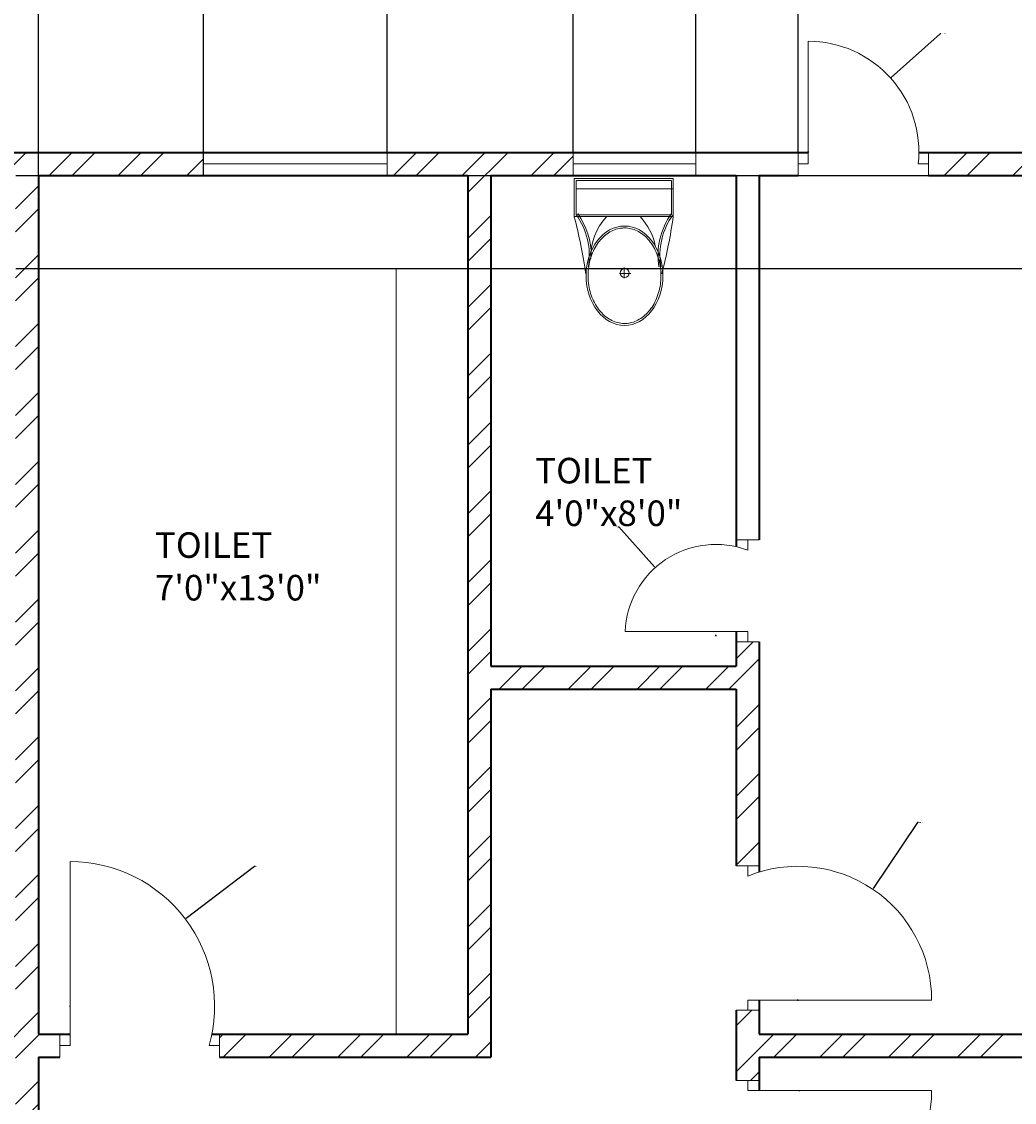
# Model space of a CAD drawing. Units: inches. Extents: x 392 to 1254, y 1207 to 2665.
# Tile 13 of 15: x 832 to 1026, y 2043 to 2255. Entities that reach past the tile are written whole.
import ezdxf

# ---------------------------------------------------------------- set-up
doc = ezdxf.new("R2010")
doc.units = ezdxf.units.IN
for name, color, linetype, lineweight in [('A-ANNO-DIMS', 2, 'Continuous', 18), ('A-AREA-IDEN', 7, 'Continuous', 18), ('A-DOOR', 3, 'Continuous', 18), ('A-FLOR-FIXT', 9, 'Continuous', 18), ('A-GLAZ', 4, 'Continuous', 18), ('A-WALL', 7, 'Continuous', 35), ('A-WALL-PATT', 252, 'Continuous', 13)]:
    doc.layers.add(name, color=color, linetype=linetype, lineweight=lineweight)
doc.styles.get("Standard").update_dxf_attribs({"font": 'arial.ttf'})
doc.dimstyles.get("Standard").update_dxf_attribs({"dimtxt": 0.18, "dimasz": 0.18, "dimexe": 0.18, "dimexo": 0.0625, "dimgap": 0.09, "dimtad": 0, "dimtih": 1, "dimtoh": 1, "dimdec": 4, "dimzin": 0, "dimdsep": 46, "dimtxsty": 'Standard', "dimcen": 0.09, "dimadec": 0, "dimazin": 0, "dimtfac": 1, "dimtdec": 4, "dimtofl": 0, "dimtmove": 0, "dimatfit": 3, "dimfxl": 1, "dimtolj": 1, "dimtzin": 0, "dimarcsym": 0})

# ---------------------------------------------------------------- blocks, each defined once
blk = doc.blocks.new('A$C31115884')
for p, q in [((257.5, 466.4), (257.5, 523.2)), ((283.1, 497.7), (223.4, 497.7)), ((0, 200), (0, 0)), ((520, 200), (0, 200)), ((10, 190), (10, 10)), ((510, 190), (10, 190)), ((510, 10), (510, 190)), ((520, 0), (520, 200)), ((510, 54.5), (0, 54.5)), ((10, 10), (510, 10)), ((0, 0), (520, 0))]:
    blk.add_line(p, q)
blk.add_circle((255.6, 496.4), 23.6)
for centre, radius, start, end in [((2777.7, -204.6), 2807, 165.4549, 171.7133), ((-294.5, 403.3), 364.7, 324.2091, 9.3499), ((-294.5, 403.3), 374.7, 324.2091, 9.3499), ((805.8, 403.3), 364.7, 170.6501, 215.7909), ((3237, 905), 2807, 188.2867, 194.5451), ((139.5, 406.2), 293.5, 315.8436, 2.6563), ((805.8, 403.3), 374.7, 179.2036, 215.7909), ((383.6, 406.2), 293.5, 190.2774, 224.1564)]:
    blk.add_arc(centre, radius, start, end)
blk.add_ellipse((256.2, 509.9), major_axis=(0, -260.7), ratio=0.772727)
blk.add_open_spline([(256.2, 259.2), (263.1, 259.2), (270, 259.7), (287.8, 262.3), (298.7, 265.1), (319.9, 273.1), (330.2, 278.4), (350.1, 291.1), (359.7, 298.7), (377.7, 315.9), (386.2, 325.5), (401.7, 346.6), (408.8, 358.1), (421.3, 382.5), (426.8, 395.5), (435.9, 422.4), (439.5, 436.4), (444.8, 465.1), (446.5, 479.7), (447.9, 509.2), (447.6, 524), (445, 553.3), (442.7, 567.8), (436.3, 596), (432.1, 609.7), (421.9, 636), (416, 648.6), (402.5, 672.1), (395, 683), (378.6, 703), (369.8, 712.1), (351.1, 728), (341.3, 734.8), (320.9, 746.2), (310.4, 750.7), (288.9, 757.3), (278, 759.4), (256, 761), (245, 760.6), (223.1, 757.2), (212.3, 754.3), (191.1, 746.1), (180.8, 740.7), (160.9, 727.8), (151.4, 720.1), (133.5, 702.7), (125.1, 693), (109.6, 671.7), (102.6, 660.2), (90.2, 635.7), (84.9, 622.7), (76, 595.6), (72.4, 581.6), (67.2, 552.9), (65.6, 538.2), (64.4, 508.8), (64.8, 494), (67.5, 464.7), (69.9, 450.2), (76.6, 422), (80.8, 408.3), (91.1, 382.2), (97.2, 369.7), (110.8, 346.3), (118.4, 335.4), (134.8, 315.6), (143.7, 306.7), (162.4, 290.9), (172.3, 284.2), (192.8, 273), (203.3, 268.6), (224.8, 262.2), (235.8, 260.2), (249.9, 259.3), (253, 259.2), (256.2, 259.2)], degree=3, knots=[0, 0, 0, 0, 0.110105, 0.110105, 0.285049, 0.285049, 0.459994, 0.459994, 0.634938, 0.634938, 0.809882, 0.809882, 0.984827, 0.984827, 1.159771, 1.159771, 1.334715, 1.334715, 1.50966, 1.50966, 1.684604, 1.684604, 1.859549, 1.859549, 2.034493, 2.034493, 2.209437, 2.209437, 2.384382, 2.384382, 2.559326, 2.559326, 2.73427, 2.73427, 2.909215, 2.909215, 3.084159, 3.084159, 3.259103, 3.259103, 3.434048, 3.434048, 3.608992, 3.608992, 3.783936, 3.783936, 3.958881, 3.958881, 4.133825, 4.133825, 4.30877, 4.30877, 4.483714, 4.483714, 4.658658, 4.658658, 4.833603, 4.833603, 5.008547, 5.008547, 5.183491, 5.183491, 5.358436, 5.358436, 5.53338, 5.53338, 5.708324, 5.708324, 5.883269, 5.883269, 6.058213, 6.058213, 6.233158, 6.233158, 6.283185, 6.283185, 6.283185, 6.283185])
blk = doc.blocks.new('WIN-24-A')
for p, q in [((0, 0), (0, 4.5)), ((0, 4.5), (0, 2.25)), ((24, 2.25), (24, 4.5)), ((24, 4.5), (24, 0)), ((0, 2.25), (24, 2.25))]:
    blk.add_line(p, q)
blk = doc.blocks.new('WIN-36')
for p, q in [((0, 0), (0, 4.5)), ((0, 4.5), (0, 2.25)), ((36, 2.25), (36, 4.5)), ((36, 4.5), (36, 0)), ((0, 2.25), (36, 2.25))]:
    blk.add_line(p, q)
blk = doc.blocks.new('*D47')
at = {"layer": 'A-ANNO-DIMS', "color": 0, "lineweight": -2, "transparency": 16777216}
for p, q in [((903.51, 2229.36), (903.51, 2297.33)), ((903.69, 2297.15), (921.29, 2297.15)), ((939.68, 2297.15), (922.08, 2297.15)), ((939.86, 2229.36), (939.86, 2297.33))]:
    blk.add_line(p, q, dxfattribs=at)
at = {"layer": 'A-ANNO-DIMS', "color": 0, "transparency": 16777216}
for points in [[(903.69, 2297.18), (903.69, 2297.12), (903.51, 2297.15)], [(939.68, 2297.18), (939.68, 2297.12), (939.86, 2297.15)]]:
    blk.add_solid(points, dxfattribs=at)
at = {"layer": 'Defpoints', "color": 0, "transparency": 16777216}
for p in [(939.86, 2297.15), (903.51, 2229.3), (939.86, 2229.3)]:
    blk.add_point(p, dxfattribs=at)
at = {"layer": 'A-ANNO-DIMS', "color": 0, "transparency": 16777216, "insert": (921.68, 2297.15), "char_height": 0.18, "attachment_point": 5}
blk.add_mtext('\\A1;36.35', dxfattribs=at)
blk = doc.blocks.new('*D48')
at = {"layer": 'A-ANNO-DIMS', "color": 0, "lineweight": -2, "transparency": 16777216}
for p, q in [((963.86, 2229.36), (963.86, 2297.33)), ((964.04, 2297.15), (973.41, 2297.15)), ((983.71, 2297.15), (974.34, 2297.15)), ((983.89, 2229.36), (983.89, 2297.33))]:
    blk.add_line(p, q, dxfattribs=at)
at = {"layer": 'A-ANNO-DIMS', "color": 0, "transparency": 16777216}
for points in [[(964.04, 2297.18), (964.04, 2297.12), (963.86, 2297.15)], [(983.71, 2297.18), (983.71, 2297.12), (983.89, 2297.15)]]:
    blk.add_solid(points, dxfattribs=at)
at = {"layer": 'Defpoints', "color": 0, "transparency": 16777216}
for p in [(983.89, 2297.15), (963.86, 2229.3), (983.89, 2229.3)]:
    blk.add_point(p, dxfattribs=at)
at = {"layer": 'A-ANNO-DIMS', "color": 0, "transparency": 16777216, "insert": (973.87, 2297.15), "char_height": 0.18, "attachment_point": 5}
blk.add_mtext('\\A1;20.026', dxfattribs=at)
blk = doc.blocks.new('*D49')
at = {"layer": 'A-ANNO-DIMS', "color": 0, "lineweight": -2, "transparency": 16777216}
for p, q in [((835.28, 2224.86), (835.28, 2297.33)), ((835.46, 2297.15), (851, 2297.15)), ((867.33, 2297.15), (851.79, 2297.15)), ((867.51, 2224.86), (867.51, 2297.33))]:
    blk.add_line(p, q, dxfattribs=at)
at = {"layer": 'A-ANNO-DIMS', "color": 0, "transparency": 16777216}
for points in [[(835.46, 2297.18), (835.46, 2297.12), (835.28, 2297.15)], [(867.33, 2297.18), (867.33, 2297.12), (867.51, 2297.15)]]:
    blk.add_solid(points, dxfattribs=at)
at = {"layer": 'Defpoints', "color": 0, "transparency": 16777216}
for p in [(867.51, 2297.15), (835.28, 2224.8), (867.51, 2224.8)]:
    blk.add_point(p, dxfattribs=at)
at = {"layer": 'A-ANNO-DIMS', "color": 0, "transparency": 16777216, "insert": (851.39, 2297.15), "char_height": 0.18, "attachment_point": 5}
blk.add_mtext('\\A1;32.23', dxfattribs=at)
blk = doc.blocks.new('*D79')
at = {"layer": 'A-ANNO-DIMS', "color": 0, "lineweight": -2, "transparency": 16777216}
for p, q in [((830.84, 2224.8), (1171.06, 2224.8)), ((1170.88, 2224.62), (1170.88, 2215.87)), ((1170.88, 2206.76), (1170.88, 2215.5)), ((830.84, 2206.58), (1171.06, 2206.58))]:
    blk.add_line(p, q, dxfattribs=at)
at = {"layer": 'A-ANNO-DIMS', "color": 0, "transparency": 16777216}
for points in [[(1170.85, 2224.62), (1170.91, 2224.62), (1170.88, 2224.8)], [(1170.85, 2206.76), (1170.91, 2206.76), (1170.88, 2206.58)]]:
    blk.add_solid(points, dxfattribs=at)
at = {"layer": 'Defpoints', "color": 0, "transparency": 16777216}
for p in [(830.78, 2224.8), (1170.88, 2224.8), (830.78, 2206.58)]:
    blk.add_point(p, dxfattribs=at)
at = {"layer": 'A-ANNO-DIMS', "color": 0, "transparency": 16777216, "insert": (1170.88, 2215.69), "char_height": 0.18, "attachment_point": 5}
blk.add_mtext('\\A1;18.22', dxfattribs=at)
blk = doc.blocks.new('*D91')
at = {"layer": 'A-ANNO-DIMS', "color": 0, "lineweight": -2, "transparency": 16777216}
for p, q in [((877.53, 2089.56), (864.13, 2079.43)), ((877.71, 2089.56), (877.53, 2089.56)), ((841.33, 2062.25), (841.51, 2062.25)), ((841.42, 2062.16), (841.42, 2062.34))]:
    blk.add_line(p, q, dxfattribs=at)
at = {"layer": 'A-ANNO-DIMS', "color": 0, "transparency": 16777216}
blk.add_solid([(864.11, 2079.45), (864.15, 2079.4), (863.99, 2079.32)], dxfattribs=at)
at = {"layer": 'Defpoints', "color": 0, "transparency": 16777216}
for p in [(863.99, 2079.32), (841.42, 2062.25)]:
    blk.add_point(p, dxfattribs=at)
at = {"layer": 'A-ANNO-DIMS', "color": 0, "transparency": 16777216, "insert": (878.12, 2089.56), "char_height": 0.18, "attachment_point": 5}
blk.add_mtext('\\A1;R28.3', dxfattribs=at)
blk = doc.blocks.new('*D95')
at = {"layer": 'A-ANNO-DIMS', "color": 0, "lineweight": -2, "transparency": 16777216}
for p, q in [((1007.25, 2098.19), (998.58, 2085.32)), ((1007.43, 2098.19), (1007.25, 2098.19)), ((983.78, 2063.47), (983.96, 2063.47)), ((983.87, 2063.38), (983.87, 2063.56))]:
    blk.add_line(p, q, dxfattribs=at)
at = {"layer": 'A-ANNO-DIMS', "color": 0, "transparency": 16777216}
blk.add_solid([(998.56, 2085.34), (998.61, 2085.3), (998.48, 2085.17)], dxfattribs=at)
at = {"layer": 'Defpoints', "color": 0, "transparency": 16777216}
for p in [(998.48, 2085.17), (983.87, 2063.47)]:
    blk.add_point(p, dxfattribs=at)
at = {"layer": 'A-ANNO-DIMS', "color": 0, "transparency": 16777216, "insert": (1007.91, 2098.19), "char_height": 0.18, "attachment_point": 5}
blk.add_mtext('\\A1;R26.16', dxfattribs=at)
blk = doc.blocks.new('*D96')
at = {"layer": 'A-ANNO-DIMS', "color": 0, "lineweight": -2, "transparency": 16777216}
for p, q in [((984.08, 2045.75), (984.26, 2045.75)), ((984.17, 2045.66), (984.17, 2045.84)), ((1006.98, 2011.23), (998.53, 2024.02)), ((1007.16, 2011.23), (1006.98, 2011.23))]:
    blk.add_line(p, q, dxfattribs=at)
at = {"layer": 'A-ANNO-DIMS', "color": 0, "transparency": 16777216}
blk.add_solid([(998.55, 2024.04), (998.5, 2024.01), (998.43, 2024.17)], dxfattribs=at)
at = {"layer": 'Defpoints', "color": 0, "transparency": 16777216}
for p in [(984.17, 2045.75), (998.43, 2024.17)]:
    blk.add_point(p, dxfattribs=at)
at = {"layer": 'A-ANNO-DIMS', "color": 0, "transparency": 16777216, "insert": (1007.71, 2011.23), "char_height": 0.18, "attachment_point": 5}
blk.add_mtext('\\A1;R25.864', dxfattribs=at)
blk = doc.blocks.new('*D97')
at = {"layer": 'A-ANNO-DIMS', "color": 0, "lineweight": -2, "transparency": 16777216}
for p, q in [((1011.67, 2252.52), (1002.14, 2243.97)), ((1011.85, 2252.52), (1011.67, 2252.52)), ((985.8, 2229.4), (985.98, 2229.4)), ((985.89, 2229.31), (985.89, 2229.49))]:
    blk.add_line(p, q, dxfattribs=at)
at = {"layer": 'A-ANNO-DIMS', "color": 0, "transparency": 16777216}
blk.add_solid([(1002.12, 2243.99), (1002.16, 2243.95), (1002, 2243.85)], dxfattribs=at)
at = {"layer": 'Defpoints', "color": 0, "transparency": 16777216}
for p in [(1002, 2243.85), (985.89, 2229.4)]:
    blk.add_point(p, dxfattribs=at)
at = {"layer": 'A-ANNO-DIMS', "color": 0, "transparency": 16777216, "insert": (1012.4, 2252.52), "char_height": 0.18, "attachment_point": 5}
blk.add_mtext('\\A1;R21.645', dxfattribs=at)
blk = doc.blocks.new('*D100')
at = {"layer": 'A-ANNO-DIMS', "color": 0, "lineweight": -2, "transparency": 16777216}
for p, q in [((948.64, 2156.02), (948.82, 2156.02)), ((948.82, 2156.02), (955.82, 2148.2)), ((967.72, 2134.81), (967.9, 2134.81)), ((967.81, 2134.72), (967.81, 2134.9))]:
    blk.add_line(p, q, dxfattribs=at)
at = {"layer": 'A-ANNO-DIMS', "color": 0, "transparency": 16777216}
blk.add_solid([(955.84, 2148.22), (955.8, 2148.18), (955.94, 2148.07)], dxfattribs=at)
at = {"layer": 'Defpoints', "color": 0, "transparency": 16777216}
for p in [(955.94, 2148.07), (967.81, 2134.81)]:
    blk.add_point(p, dxfattribs=at)
at = {"layer": 'A-ANNO-DIMS', "color": 0, "transparency": 16777216, "insert": (948.16, 2156.02), "char_height": 0.18, "attachment_point": 5}
blk.add_mtext('\\A1;R17.79', dxfattribs=at)

msp = doc.modelspace()

# ---------------------------------------------------------------- hatches: boundary and pattern name
at = {"layer": 'A-WALL-PATT'}
h = msp.add_hatch(dxfattribs=at)
h.set_pattern_fill('ANSI32', color=256)
h.paths.add_polyline_path([(579.5309, 2227.0453), (579.5309, 2229.2953), (541.2807, 2229.2953), (541.2807, 2182.3091), (545.7807, 2182.3091), (545.7807, 2224.7953), (579.5309, 2224.7953)])
h.paths.add_polyline_path([(655.4442, 2229.2953), (627.5309, 2229.2953), (627.5309, 2224.7953), (655.4442, 2224.7953), (655.4442, 2227.0453)])
h.paths.add_polyline_path([(703.0758, 2229.2953), (678.5257, 2229.2953), (678.5257, 2227.0453), (678.5257, 2224.7953), (689.7807, 2224.7953), (689.7807, 2158.6973), (694.2807, 2158.6973), (694.2807, 2224.7953), (703.0758, 2224.7953)])
h.paths.add_polyline_path([(768.5767, 2229.2953), (727.0758, 2229.2953), (727.0758, 2224.7953), (742.2807, 2224.7953), (742.2807, 2128.7953), (694.2807, 2128.7953), (694.2807, 2134.0554), (689.7807, 2134.0554), (689.7807, 2090.2854), (694.2807, 2090.2854), (694.2807, 2124.2953), (742.2807, 2124.2953), (742.2807, 2052.2953), (795.2124, 2052.2953), (795.2124, 2054.5453), (795.2124, 2056.7953), (746.7807, 2056.7953), (746.7807, 2224.7953), (768.5767, 2224.7953)])
h.paths.add_polyline_path([(867.5089, 2229.2953), (804.5767, 2229.2953), (804.5767, 2224.7953), (830.7807, 2224.7953), (830.7807, 2056.7953), (826.9066, 2056.7953), (826.9066, 2052.2953), (830.7807, 2052.2953), (830.7807, 1886.6777, -0.01766664), (830.8602, 1884.2953), (835.0818, 1884.2953, -0.04411348), (835.2807, 1889.9369), (835.2807, 2052.2953), (839.418, 2052.2953), (839.418, 2056.7953), (835.2807, 2056.7953), (835.2807, 2224.7953), (867.5089, 2224.7953)])
h.paths.add_polyline_path([(939.8604, 2229.2953), (903.5089, 2229.2953), (903.5089, 2227.0453), (903.5089, 2224.7953), (919.2807, 2224.7953), (919.2807, 2056.7953), (870.6499, 2056.7953), (870.6499, 2052.2953), (923.7807, 2052.2953), (923.7807, 2124.2953), (971.7807, 2124.2953), (971.7807, 2089.7112), (974.0307, 2089.7112), (976.2807, 2089.7112), (976.2807, 2133.56), (974.0307, 2133.56), (971.7807, 2133.56), (971.7807, 2128.7953), (923.7807, 2128.7953), (923.7807, 2224.7953), (939.8604, 2224.7953)])
h.paths.add_polyline_path([(1124.7807, 2229.2953), (1009.403, 2229.2953), (1009.403, 2224.7953), (1120.2807, 2224.7953), (1120.2807, 2184.7605), (1124.7807, 2184.7605)])
h.paths.add_polyline_path([(1124.7807, 2124.7605), (1120.2807, 2124.7605), (1120.2807, 2056.7953), (976.2807, 2056.7953), (976.2807, 2061.471), (971.7807, 2061.471), (971.7807, 2047.7483), (974.0307, 2047.7483), (976.2807, 2047.7483), (976.2807, 2052.2953), (1120.2807, 2052.2953), (1120.2807, 1992.457), (1124.7807, 1992.457)])
h.paths.add_polyline_path([(1124.7807, 1932.457), (1122.5307, 1932.457), (1120.2807, 1932.457), (1120.2807, 1884.2953), (976.2807, 1884.2953), (976.2807, 2019.9536), (971.7807, 2019.9536), (971.7807, 1884.2953), (869.0911, 1884.2953), (869.0911, 1879.7953), (971.7807, 1879.7953), (1013.7807, 1879.7953), (1013.7807, 1831.7953), (971.7807, 1831.7953), (971.7807, 1822.3831), (974.0307, 1822.3831), (976.2807, 1822.3831), (976.2807, 1827.2953), (1013.7807, 1827.2953), (1025.6191, 1827.2953), (1025.6191, 1829.5453), (1025.6191, 1831.7953), (1018.2807, 1831.7953), (1018.2807, 1879.7953), (1120.2807, 1879.7953), (1120.2807, 1866.9192), (1124.7807, 1866.9192)])
h.paths.add_polyline_path([(1124.7807, 1842.9192), (1122.5307, 1842.9192), (1120.2807, 1842.9192), (1120.2807, 1831.7953), (1050.2021, 1831.7953), (1050.2021, 1827.2953), (1120.2807, 1827.2953), (1120.2807, 1781.4559), (1124.7807, 1781.4559)])
h.paths.add_polyline_path([(976.2807, 1790.8718), (971.7807, 1790.8718), (971.7807, 1648.3339), (976.2807, 1648.3339), (976.2807, 1654.7953), (1120.2807, 1654.7953), (1120.2807, 1626.3807), (1124.7807, 1626.3807), (1124.7807, 1721.4559), (1120.2807, 1721.4559), (1120.2807, 1659.2953), (976.2807, 1659.2953)])
h.paths.add_polyline_path([(1124.7807, 1566.3807), (1120.2807, 1566.3807), (1120.2807, 1486.7953), (1101.07, 1486.7953), (1101.07, 1482.2953), (1124.7807, 1482.2953)])
h.paths.add_polyline_path([(1041.07, 1484.5453), (1041.07, 1486.7953), (1006.2807, 1486.7953), (1006.2807, 1484.5453), (1006.2807, 1482.2953), (1041.07, 1482.2953)])
h.paths.add_polyline_path([(976.2807, 1617.5497), (974.0307, 1617.5497), (971.7807, 1617.5497), (971.7807, 1599.2953), (965.8041, 1599.2953), (965.8041, 1594.7953), (971.7807, 1594.7953), (971.7807, 1486.7953), (954.1249, 1486.7953), (954.1249, 1482.2953), (981.5717, 1482.2953), (981.5717, 1484.5453), (981.5717, 1486.7953), (976.2807, 1486.7953)])
h.paths.add_polyline_path([(930.1249, 1486.7953), (887.7807, 1486.7953), (887.7807, 1594.7953), (941.9141, 1594.7953), (941.9141, 1597.0453), (941.9141, 1599.2953), (887.7807, 1599.2953), (887.7807, 1659.2953), (863.5916, 1659.2953), (863.5916, 1654.7953), (883.2807, 1654.7953), (883.2807, 1438.7953), (782.7807, 1438.7953), (782.7807, 1486.7953), (782.7807, 1654.7953), (800.1309, 1654.7953), (800.1309, 1657.0453), (800.1309, 1659.2953), (778.2807, 1659.2953), (778.2807, 1599.2953), (721.7333, 1599.2953), (721.7333, 1597.0453), (721.7333, 1594.7953), (778.2807, 1594.7953), (778.2807, 1486.7953), (729.598, 1486.7953), (729.598, 1482.2953), (753.2885, 1482.2953), (753.2885, 1410.2953), (922.9852, 1410.2953), (922.9852, 1482.2953), (930.1249, 1482.2953)])
h.paths.add_polyline_path([(918.4852, 1482.2953), (918.4852, 1414.7953), (757.7885, 1414.7953), (757.7885, 1482.2953), (778.2807, 1482.2953), (778.2807, 1434.2953), (782.7807, 1434.2953), (887.7807, 1434.2953), (887.7807, 1438.7953), (887.7807, 1482.2953)], flags=16)
h.paths.add_polyline_path([(694.2807, 1594.7953), (700.4169, 1594.7953), (700.4169, 1597.0453), (700.4169, 1599.2953), (694.2807, 1599.2953), (694.2807, 1617.7503), (692.0307, 1617.7503), (689.7807, 1617.7503), (689.7807, 1486.7953), (682.7672, 1486.7953), (682.7672, 1482.2953), (705.598, 1482.2953), (705.598, 1484.5453), (705.598, 1486.7953), (694.2807, 1486.7953)])
h.paths.add_polyline_path([(545.7807, 1654.7953), (689.7807, 1654.7953), (689.7807, 1649.7691), (694.2807, 1649.7691), (694.2807, 1789.3981), (692.0307, 1789.3981), (689.7807, 1789.3981), (689.7807, 1659.2953), (545.7807, 1659.2953), (545.7807, 1714.4681), (543.5307, 1714.4681), (541.2807, 1714.4681), (541.2807, 1482.2953), (567.0628, 1482.2953), (567.0628, 1484.5453), (567.0628, 1486.7953), (545.7807, 1486.7953)])
h.paths.add_polyline_path([(545.7807, 1827.2953), (620.2247, 1827.2953), (620.2247, 1829.5453), (620.2247, 1831.7953), (545.7807, 1831.7953), (545.7807, 1846.8518), (541.2807, 1846.8518), (541.2807, 1774.4681), (545.7807, 1774.4681)])
h.paths.add_polyline_path([(797.0944, 1884.2953), (694.2807, 1884.2953), (694.2807, 2019.0288), (692.0307, 2019.0288), (689.7807, 2019.0288), (689.7807, 1884.2953), (545.7807, 1884.2953), (545.7807, 1951.8244), (541.2807, 1951.8244), (541.2807, 1870.8518), (543.5307, 1870.8518), (545.7807, 1870.8518), (545.7807, 1879.7953), (647.7807, 1879.7953), (647.7807, 1831.7953), (642.6413, 1831.7953), (642.6413, 1827.2953), (652.2807, 1827.2953), (689.7807, 1827.2953), (689.7807, 1821.0531), (694.2807, 1821.0531), (694.2807, 1831.7953), (652.2807, 1831.7953), (652.2807, 1879.7953), (797.0944, 1879.7953), (797.0944, 1882.0453)])
h.paths.add_polyline_path([(545.7807, 2122.3091), (541.2807, 2122.3091), (541.2807, 2011.8244), (543.5307, 2011.8244), (545.7807, 2011.8244), (545.7807, 2052.2953), (689.7807, 2052.2953), (689.7807, 2048.2048), (694.2807, 2048.2048), (694.2807, 2061.3129), (692.0307, 2061.3129), (689.7807, 2061.3129), (689.7807, 2056.7953), (545.7807, 2056.7953)])

# ---------------------------------------------------------------- linework, layer by layer
at = {"layer": 'A-DOOR'}
for p, q in [((985.8869, 2227.0453), (985.8869, 2251.0453)), ((983.8869, 2224.7953), (983.8869, 2229.2953)), ((983.8869, 2229.2953), (983.8869, 2227.0453)), ((1009.403, 2229.2953), (1009.403, 2224.7953)), ((983.8869, 2227.0453), (985.8869, 2227.0453)), ((1009.403, 2227.0453), (1007.403, 2227.0453)), ((1009.403, 2224.7953), (1009.403, 2227.0453)), ((971.7807, 2153.4791), (976.2807, 2153.4791)), ((976.2807, 2153.4791), (974.0307, 2153.4791)), ((974.0307, 2153.4791), (974.0307, 2151.4791)), ((974.0307, 2135.56), (950.0307, 2135.56)), ((974.0307, 2133.56), (974.0307, 2135.56)), ((971.7807, 2133.56), (976.2807, 2133.56)), ((976.2807, 2133.56), (974.0307, 2133.56)), ((841.418, 2054.5453), (841.418, 2090.5453)), ((976.2807, 2089.7112), (971.7807, 2089.7112)), ((971.7807, 2089.7112), (974.0307, 2089.7112)), ((974.0307, 2089.7112), (974.0307, 2087.7112)), ((974.0307, 2061.471), (974.0307, 2063.471)), ((974.0307, 2063.471), (1010.0307, 2063.471)), ((976.2807, 2061.471), (971.7807, 2061.471)), ((971.7807, 2061.471), (974.0307, 2061.471)), ((839.418, 2052.2953), (839.418, 2056.7953)), ((839.418, 2056.7953), (839.418, 2054.5453)), ((870.6499, 2056.7953), (870.6499, 2052.2953)), ((839.418, 2054.5453), (841.418, 2054.5453)), ((870.6499, 2054.5453), (868.6499, 2054.5453)), ((870.6499, 2052.2953), (870.6499, 2054.5453)), ((976.2807, 2047.7483), (971.7807, 2047.7483)), ((971.7807, 2047.7483), (974.0307, 2047.7483)), ((974.0307, 2047.7483), (974.0307, 2045.7483)), ((974.0307, 2045.7483), (1010.0307, 2045.7483))]:
    msp.add_line(p, q, dxfattribs=at)
for centre, radius, start, end in [((985.8869, 2229.4007), 21.6447, 353.752763, 90), ((967.8067, 2134.8115), 17.7917, 69.523338, 177.589031), ((841.418, 2062.2456), 28.2997, 344.210903, 90), ((983.8698, 2063.471), 26.161, 360, 112.092096), ((984.167, 2045.7483), 25.8637, 246.92657, 0)]:
    msp.add_arc(centre, radius, start, end, dxfattribs=at)
at = {"layer": 'A-FLOR-FIXT'}
for p, q in [((835.2807, 2206.5771), (905.2243, 2206.5771)), ((905.2243, 2206.5771), (905.2243, 2056.7953))]:
    msp.add_line(p, q, dxfattribs=at)
at = {"layer": 'A-WALL'}
for p, q in [((676.5257, 2229.2953), (985.8869, 2229.2953)), ((1007.5313, 2229.2953), (1124.7807, 2229.2953)), ((835.2807, 2224.7953), (835.2807, 2056.7953)), ((835.2807, 2224.7953), (919.2807, 2224.7953)), ((919.2807, 2224.7953), (919.2807, 2056.7953)), ((923.7807, 2224.7953), (923.7807, 2128.7953)), ((923.7807, 2224.7953), (971.7807, 2224.7953)), ((971.7807, 2224.7953), (971.7807, 2152.1538)), ((976.2807, 2224.7953), (976.2807, 2153.4791)), ((976.2807, 2224.7953), (983.8869, 2224.7953)), ((1009.403, 2224.7953), (1120.2807, 2224.7953)), ((971.7807, 2135.56), (971.7807, 2128.7953)), ((976.2807, 2133.56), (976.2807, 2088.507)), ((923.7807, 2128.7953), (971.7807, 2128.7953)), ((923.7807, 2124.2953), (971.7807, 2124.2953)), ((923.7807, 2124.2953), (923.7807, 2052.2953)), ((971.7807, 2124.2953), (971.7807, 2089.7112)), ((976.2807, 2063.471), (976.2807, 2056.7953)), ((971.7807, 2061.471), (971.7807, 2047.7483)), ((835.2807, 2056.7953), (841.418, 2056.7953)), ((869.1879, 2056.7953), (919.2807, 2056.7953)), ((976.2807, 2056.7953), (1120.2807, 2056.7953)), ((835.2807, 2052.2953), (835.2807, 1889.9369)), ((835.2807, 2052.2953), (839.418, 2052.2953)), ((870.6499, 2052.2953), (923.7807, 2052.2953)), ((976.2807, 2052.2953), (1120.2807, 2052.2953)), ((976.2807, 2052.2953), (976.2807, 2045.7483))]:
    msp.add_line(p, q, dxfattribs=at)

# ---------------------------------------------------------------- block references
at = {"layer": 'A-FLOR-FIXT', "xscale": 0.0372717239612423, "yscale": 0.0372717239612423, "zscale": 0.0372717239612423, "rotation": 180}
msp.add_blockref('A$C31115884', (959.4737, 2224.176), dxfattribs=at)
at = {"layer": 'A-GLAZ', "extrusion": (0, 0, -1), "zscale": -1}
for name, p in [('WIN-36', (-903.5086, 2224.795)), ('WIN-24-A', (-963.8602, 2224.795))]:
    msp.add_blockref(name, p, dxfattribs=at)

# ---------------------------------------------------------------- texts
at = {"layer": 'A-AREA-IDEN', "char_height": 5, "attachment_point": 1}
for s, width, insert in [('TOILET\\P4\'0"x8\'0"', 118.028233, (932.4524, 2169.5331)), ('TOILET\\P7\'0"x13\'0"', 180.647683, (858.0433, 2154.9695))]:
    msp.add_mtext_dynamic_manual_height_columns(s, width=width, gutter_width=12.5, heights=[0], dxfattribs=dict(at, insert=insert))

# ---------------------------------------------------------------- dimensions: what is measured, and where the dimension line sits
at = {"layer": 'A-ANNO-DIMS'}
for base, p1, p2, override, picture, middle in [((867.5089, 2297.1453), (835.2807, 2224.7953), (867.5089, 2224.7953), {"dimdec": 2, "dimlfac": 1, "dimrnd": 0, "dimzin": 0, "dimdsep": 46, "dimlunit": 2}, '*D49', (851.3948, 2297.1453)), ((939.8604, 2297.1453), (903.5089, 2229.2953), (939.8604, 2229.2953), {"dimdec": 2, "dimlfac": 1, "dimrnd": 0, "dimzin": 0, "dimdsep": 46, "dimlunit": 2}, '*D47', (921.6846, 2297.1453)), ((983.88686, 2297.14532), (963.86038, 2229.29532), (983.88686, 2229.29532), {"dimdec": 3, "dimlfac": 1, "dimrnd": 0, "dimzin": 0, "dimdsep": 46, "dimlunit": 2}, '*D48', (973.87362, 2297.14532))]:
    dim = msp.add_linear_dim(base=base, p1=p1, p2=p2, dimstyle='Standard', override=override, dxfattribs=at)
    dim.commit()
    dim.dimension.update_dxf_attribs({"geometry": picture, "text_midpoint": middle})
for center, mpoint, override, picture, middle in [((985.8869, 2229.4007), (1002.0031, 2243.8491), {"dimdec": 3, "dimlfac": 1, "dimrnd": 0, "dimzin": 0, "dimdsep": 46, "dimlunit": 2}, '*D97', (1012.4033, 2252.5182)), ((967.8067, 2134.8115), (955.9396, 2148.0674), {"dimdec": 2, "dimlfac": 1, "dimrnd": 0, "dimzin": 0, "dimdsep": 46, "dimlunit": 2}, '*D100', (948.1594, 2156.021)), ((983.8698, 2063.471), (998.4812, 2085.1712), {"dimdec": 2, "dimlfac": 1, "dimrnd": 0, "dimzin": 0, "dimdsep": 46, "dimlunit": 2}, '*D95', (1007.9078, 2098.1914)), ((841.418, 2062.2456), (863.988, 2079.318), {"dimdec": 1, "dimlfac": 1, "dimrnd": 0, "dimzin": 0, "dimdsep": 46, "dimlunit": 2}, '*D91', (878.12, 2089.5615)), ((984.167, 2045.7483), (998.4282, 2024.1717), {"dimdec": 3, "dimlfac": 1, "dimrnd": 0, "dimzin": 0, "dimdsep": 46, "dimlunit": 2}, '*D96', (1007.7143, 2011.2257))]:
    dim = msp.add_radius_dim(center=center, mpoint=mpoint, dimstyle='Standard', override=override, dxfattribs=at)
    dim.commit()
    dim.dimension.update_dxf_attribs({"geometry": picture, "text_midpoint": middle, "dimtype": 164})
dim = msp.add_linear_dim(base=(1170.8807, 2224.7953), p1=(830.7807, 2206.5771), p2=(830.7807, 2224.7953), angle=90, dimstyle='Standard', override={"dimdec": 2, "dimlfac": 1, "dimrnd": 0, "dimzin": 0, "dimdsep": 46, "dimlunit": 2}, dxfattribs=at)
dim.commit()
dim.dimension.update_dxf_attribs({"geometry": '*D79', "text_midpoint": (1170.8807, 2215.6862)})

doc.saveas('drawing.dxf')
